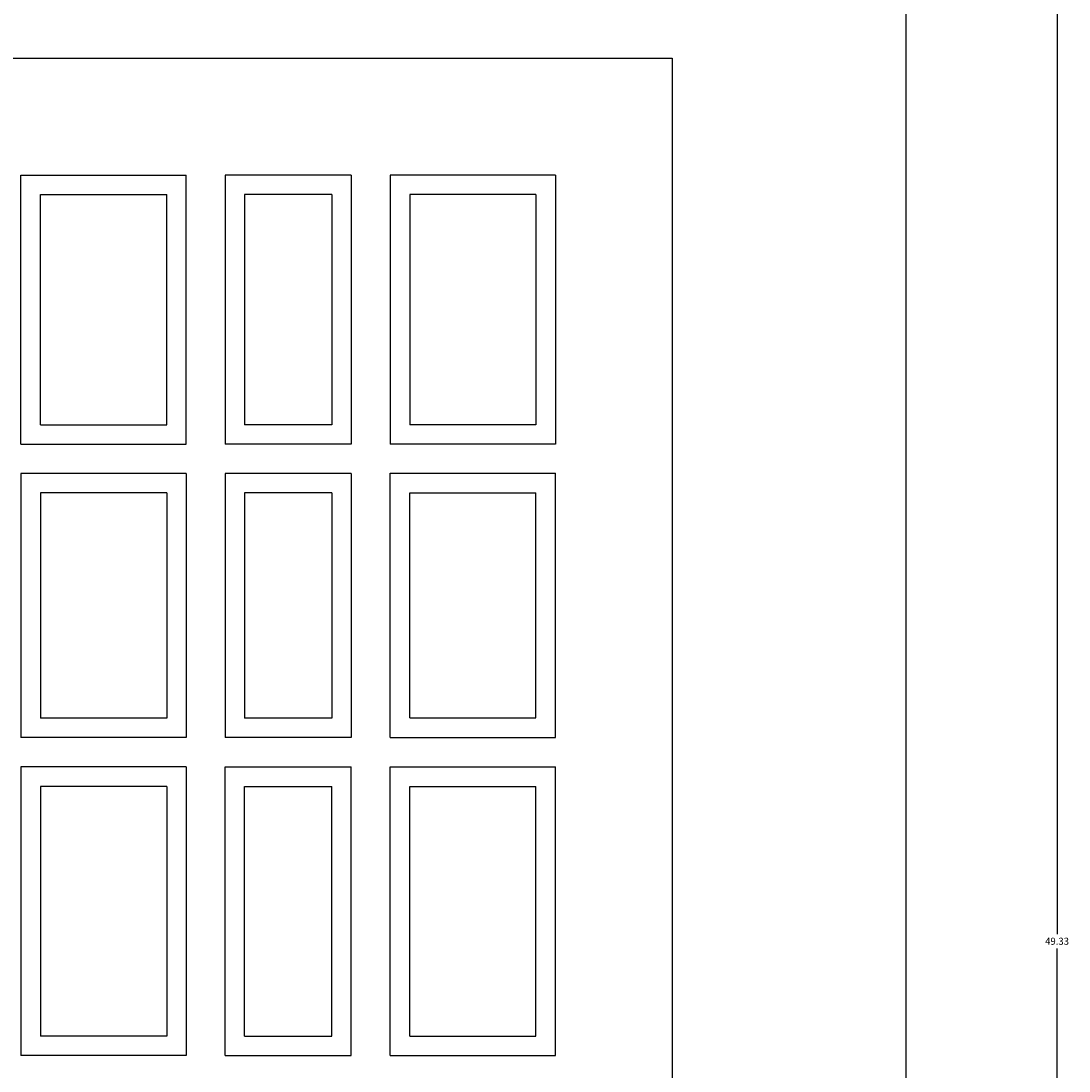
# Model space of a CAD drawing. Units: inches. Extents: x 12532.3 to 12594.9, y 6967.5 to 7063.
# Tile 5 of 9: x 12566.2 to 12593.1, y 6992.9 to 7019.9. Entities that reach past the tile are written whole.
import ezdxf

# ---------------------------------------------------------------- set-up
doc = ezdxf.new("R2010")
doc.units = ezdxf.units.IN
doc.header["$MEASUREMENT"] = 0
doc.header["$PDMODE"] = 98
doc.layers.add('A-ANNO-DIMS', color=2, linetype='Continuous', lineweight=18)
doc.layers.add('A-DOOR', color=4, linetype='Continuous', lineweight=25)
doc.styles.get("Standard").update_dxf_attribs({"font": 'arial.ttf'})
doc.dimstyles.get("Standard").update_dxf_attribs({"dimtxt": 0.18, "dimasz": 0.18, "dimexe": 0.18, "dimexo": 0.0625, "dimgap": 0.09, "dimtad": 0, "dimtih": 1, "dimtoh": 1, "dimdec": 4, "dimzin": 0, "dimdsep": 46, "dimtxsty": 'Standard', "dimcen": 0.09, "dimadec": 0, "dimazin": 0, "dimtfac": 1, "dimtdec": 4, "dimtofl": 0, "dimtmove": 0, "dimatfit": 3, "dimfxl": 1, "dimtolj": 1, "dimtzin": 0, "dimarcsym": 0})

# ---------------------------------------------------------------- blocks, each defined once
blk = doc.blocks.new('DOOR-PANEL-4_2x6_9')
for p, q in [((4.241, 6.908), (0, 6.908)), ((0, 6.908), (0, 0)), ((4.241, 6.908), (4.241, 0)), ((3.741, 6.408), (0.5, 6.408)), ((0.5, 6.408), (0.5, 0.5)), ((3.741, 6.408), (3.741, 0.5)), ((3.741, 0.5), (0.5, 0.5)), ((4.241, 0), (0, 0))]:
    blk.add_line(p, q)
blk = doc.blocks.new('DOOR-PANEL-4_2x6_8')
for p, q in [((4.241, 6.78), (0, 6.78)), ((0, 6.78), (0, 0)), ((4.241, 6.78), (4.241, 0)), ((3.741, 6.28), (0.5, 6.28)), ((0.5, 6.28), (0.5, 0.5)), ((3.741, 6.28), (3.741, 0.5)), ((3.741, 0.5), (0.5, 0.5)), ((4.241, 0), (0, 0))]:
    blk.add_line(p, q)
blk = doc.blocks.new('DOOR-PANEL-4_2x7_4')
for p, q in [((4.241, 7.408), (0, 7.408)), ((0, 7.408), (0, 0)), ((4.241, 7.408), (4.241, 0)), ((3.741, 6.908), (0.5, 6.908)), ((0.5, 6.908), (0.5, 0.5)), ((3.741, 6.908), (3.741, 0.5)), ((3.741, 0.5), (0.5, 0.5)), ((4.241, 0), (0, 0))]:
    blk.add_line(p, q)
blk = doc.blocks.new('DOOR-PANEL-3_2x7_4')
for p, q in [((0, 0), (0, 7.408)), ((0, 7.408), (3.24, 7.408)), ((3.24, 0), (3.24, 7.408)), ((0.5, 0.5), (0.5, 6.908)), ((0.5, 6.908), (2.74, 6.908)), ((2.74, 0.5), (2.74, 6.908)), ((0.5, 0.5), (2.74, 0.5)), ((0, 0), (3.24, 0))]:
    blk.add_line(p, q)
blk = doc.blocks.new('DOOR-PANEL-3_2x6_8')
for p, q in [((0, 6.78), (0, 0)), ((3.24, 6.78), (0, 6.78)), ((3.24, 6.78), (3.24, 0)), ((0.5, 6.28), (0.5, 0.5)), ((2.74, 6.28), (0.5, 6.28)), ((2.74, 6.28), (2.74, 0.5)), ((2.74, 0.5), (0.5, 0.5)), ((3.24, 0), (0, 0))]:
    blk.add_line(p, q)
blk = doc.blocks.new('DOOR-PANEL-3_2x6_9')
for p, q in [((0, 0), (0, 6.908)), ((0, 6.908), (3.24, 6.908)), ((3.24, 0), (3.24, 6.908)), ((0.5, 0.5), (0.5, 6.408)), ((0.5, 6.408), (2.74, 6.408)), ((2.74, 0.5), (2.74, 6.408)), ((0.5, 0.5), (2.74, 0.5)), ((0, 0), (3.24, 0))]:
    blk.add_line(p, q)
blk = doc.blocks.new('*D32')
at = {"layer": 'A-ANNO-DIMS', "color": 0, "lineweight": -2, "transparency": 16777216}
for p, q in [((12588.956, 7020.929), (12592.954, 7020.929)), ((12592.774, 7020.749), (12592.774, 6996.445)), ((12592.774, 6971.777), (12592.774, 6996.081)), ((12588.956, 6971.597), (12592.954, 6971.597))]:
    blk.add_line(p, q, dxfattribs=at)
at = {"layer": 'A-ANNO-DIMS', "color": 0, "transparency": 16777216}
for points in [[(12592.744, 7020.749), (12592.804, 7020.749), (12592.774, 7020.929)], [(12592.744, 6971.777), (12592.804, 6971.777), (12592.774, 6971.597)]]:
    blk.add_solid(points, dxfattribs=at)
at = {"layer": 'Defpoints', "color": 0, "transparency": 16777216}
for p in [(12588.894, 7020.929), (12592.774, 7020.929), (12588.894, 6971.597)]:
    blk.add_point(p, dxfattribs=at)
at = {"layer": 'A-ANNO-DIMS', "color": 0, "transparency": 16777216, "insert": (12592.774, 6996.263), "char_height": 0.18, "attachment_point": 5}
blk.add_mtext('\\A1;49.33', dxfattribs=at)

msp = doc.modelspace()

# ---------------------------------------------------------------- linework, layer by layer
at = {"layer": 'A-DOOR'}
msp.add_lwpolyline([(12536.4501, 7020.9287), (12588.894, 7020.9287), (12588.894, 6971.5968), (12536.4501, 6971.5968)], close=True, dxfattribs=at)
for points in [[(12542.4501, 7018.9287), (12582.894, 7018.9287)], [(12582.894, 7018.9287), (12582.894, 6973.5968)]]:
    msp.add_lwpolyline(points, dxfattribs=at)

# ---------------------------------------------------------------- block references
at = {"layer": 'A-DOOR', "rotation": 180}
for name, p in [('DOOR-PANEL-4_2x6_9', (12570.4129, 7015.9287)), ('DOOR-PANEL-3_2x6_9', (12574.6531, 7015.9287)), ('DOOR-PANEL-4_2x6_8', (12579.8941, 7008.2739)), ('DOOR-PANEL-4_2x7_4', (12579.8941, 7000.738))]:
    msp.add_blockref(name, p, dxfattribs=at)
at = {"layer": 'A-DOOR'}
for name, p in [('DOOR-PANEL-4_2x6_9', (12575.6532, 7009.021)), ('DOOR-PANEL-4_2x6_8', (12566.1719, 7001.493)), ('DOOR-PANEL-3_2x6_8', (12571.4129, 7001.493)), ('DOOR-PANEL-4_2x7_4', (12566.1719, 6993.33)), ('DOOR-PANEL-3_2x7_4', (12571.4129, 6993.33))]:
    msp.add_blockref(name, p, dxfattribs=at)

# ---------------------------------------------------------------- dimensions: what is measured, and where the dimension line sits
at = {"layer": 'A-ANNO-DIMS'}
dim = msp.add_linear_dim(base=(12592.774, 7020.9287), p1=(12588.894, 6971.5968), p2=(12588.894, 7020.9287), angle=90, dimstyle='Standard', override={"dimdec": 2, "dimlfac": 1, "dimrnd": 0, "dimzin": 0, "dimdsep": 46, "dimlunit": 2}, dxfattribs=at)
dim.commit()
dim.dimension.update_dxf_attribs({"geometry": '*D32', "text_midpoint": (12592.774, 6996.2627)})

doc.saveas('drawing.dxf')
